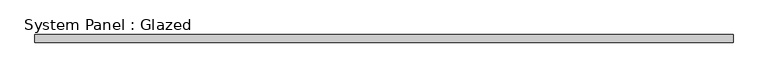
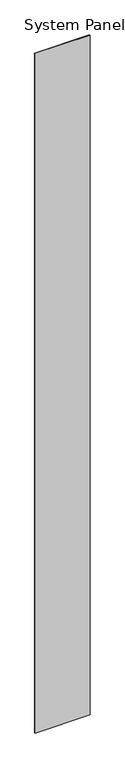
"""IFC4 building model written with IfcOpenShell, lengths in millimetres: plate geometry, System Panel : Glazed."""

from ifc_helpers import new_model, si_unit, origin, origin_with_axes, place, context, project, spatial, polyline, outline, extrude, source, transform, mapped, element, save


def system_panel_glazed_e0938204(model_context):
    return source(origin(), model_context, "Body", "SweptSolid", [
        extrude(outline(polyline([(1112.3083333, 19.05), (-1112.3083333, 19.05), (-1112.3083333, 44.45), (1112.3083333, 44.45), (1112.3083333, 19.05)])), origin_with_axes(), (0.0, 0.0, 1.0), 29133.8),
    ])


if __name__ == "__main__":
    model = new_model("IFC4")
    model_context = context("Model", 3, world=origin())
    ifc_project = project(units=[si_unit("LENGTHUNIT", "METRE", prefix="MILLI")], contexts=[model_context])
    site = spatial("IfcSite", under=ifc_project)
    building = spatial("IfcBuilding", under=site)
    placement = place(None, origin())
    system_panel_glazed_shape = system_panel_glazed_e0938204(model_context)
    element("IfcPlate", 1, ObjectType="System Panel : Glazed", at=placement, inside=building, context=model_context, shape_type="MappedRepresentation", body=[
        mapped(system_panel_glazed_shape, transform((0.0, 0.0, 0.0), x_axis=(1.0, 0.0, 0.0), y_axis=(0.0, 1.0, 0.0), z_axis=(0.0, 0.0, 1.0))),
    ])
    save(model, "model.ifc")

# Revit data of these elements
# Type "System Panel : Glazed"
#   Construction Type Id = "GSP4R"
#   Analytic Construction = "1/8 in Pilkington single glazing"
#   Visual Light Transmittance = 0.9
#   Solar Heat Gain Coefficient = 0.86
#   Heat Transfer Coefficient (U) = 1.18115 BTU/(h·ft²·°F)
# Element 1 (IfcPlate, "System Panel : Glazed")
#   Materials on its faces: "Glass"
# Materials
#   "Glass": class "Glass", colour RGB 0 128 192, transparency 0.75, Description = "Soda Lime Glass", Cost = 0
